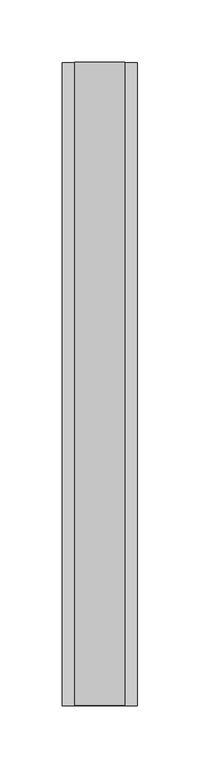
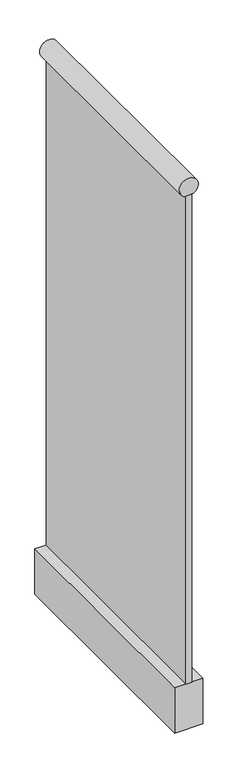
"""IFC4 building model written with IfcOpenShell, lengths in millimetres: railing geometry."""

from ifc_helpers import new_model, si_unit, point, frame, frame_2d, origin, place, context, project, spatial, polyline, circle_curve, trimmed, segment, composite_curve, outline, extrude, source, transform, mapped, element, save


def railing_3627d9a0(model_context):
    return source(origin(), model_context, "Body", "SweptSolid", [
        extrude(outline(composite_curve([segment(trimmed(circle_curve(frame_2d((8465.3205081, -1533.8712297)), 20.0), [point((8448.0, -1523.8712297))], [point((8448.0, -1543.8712297))], False, "CARTESIAN"), True, "CONTINUOUS"), segment(polyline([(8448.0, -1543.8712297), (8448.0, -1523.8712297)]), True, "CONTINUOUS")], self_intersect=False)), frame((0.0, -7637.0014262, 0.0), z_axis=(0.0, 1.0, 0.0), x_axis=(0.0, 0.0, 1.0)), (0.0, 0.0, 1.0), 515.0),
        extrude(outline(polyline([(-1527.8712297, -7637.0014262), (-1539.8712297, -7637.0014262), (-1539.8712297, -7122.0014262), (-1527.8712297, -7122.0014262), (-1527.8712297, -7637.0014262)])), frame((0.0, 0.0, 7350.0), z_axis=(0.0, 0.0, 1.0), x_axis=(1.0, 0.0, 0.0)), (0.0, 0.0, 1.0), 1098.0),
        extrude(outline(polyline([(-1503.8712297, -7637.0014262), (-1563.8712297, -7637.0014262), (-1563.8712297, -7122.0014262), (-1503.8712297, -7122.0014262), (-1503.8712297, -7637.0014262)])), frame((0.0, 0.0, 7248.0), z_axis=(0.0, 0.0, 1.0), x_axis=(1.0, 0.0, 0.0)), (0.0, 0.0, 1.0), 102.0),
    ])


if __name__ == "__main__":
    model = new_model("IFC4")
    model_context = context("Model", 3, world=origin())
    ifc_project = project(units=[si_unit("LENGTHUNIT", "METRE", prefix="MILLI")], contexts=[model_context])
    site = spatial("IfcSite", under=ifc_project)
    building = spatial("IfcBuilding", under=site)
    placement = place(None, origin())
    railing_shape = railing_3627d9a0(model_context)
    element("IfcRailing", 1, at=placement, inside=building, context=model_context, shape_type="MappedRepresentation", body=[
        mapped(railing_shape, transform((0.0, 0.0, 0.0), x_axis=(1.0, 0.0, 0.0), y_axis=(0.0, 1.0, 0.0), z_axis=(0.0, 0.0, 1.0))),
    ])
    save(model, "model.ifc")

# Revit data of these elements
# Element 1 (IfcRailing)
#   Materials on its faces: "Metal - Aluminum"
# Materials
#   "Metal - Aluminum": colour RGB 247 247 247, transparency 0, Cost = 0
